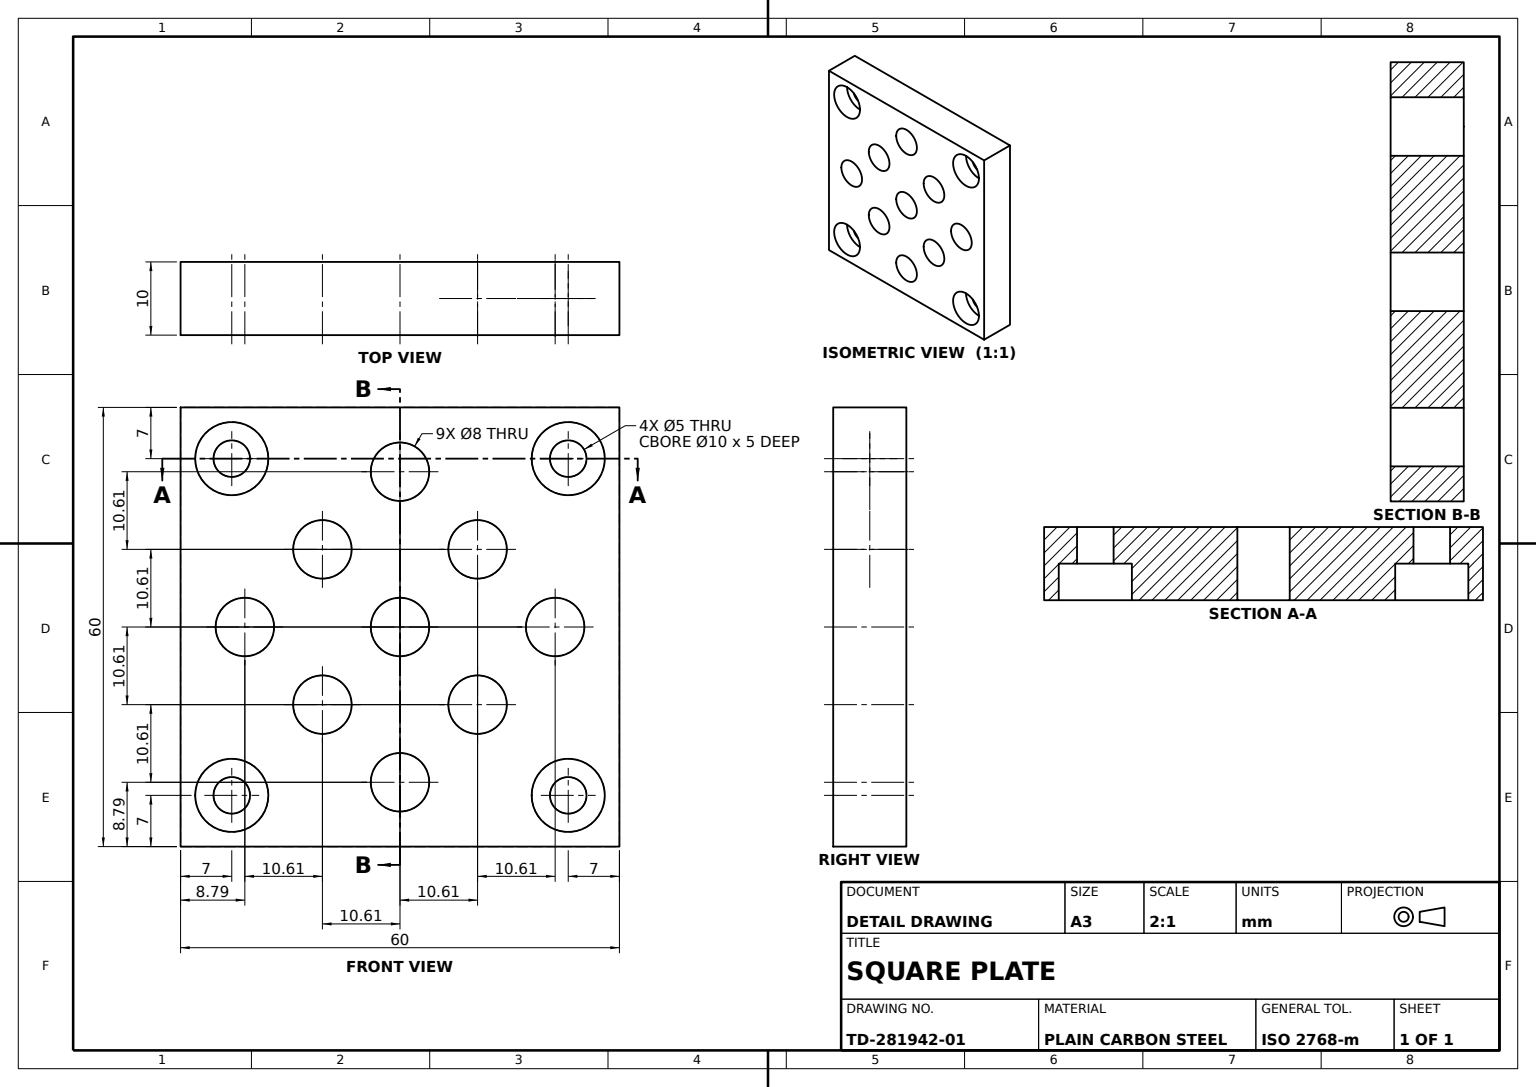
SolidWorks part; units mm, degrees
material "Plain Carbon Steel"
ref_plane "Front Plane" through (0, 0, 0) normal (0, 0, 1) x (1, 0, 0)
ref_plane "Top Plane" through (0, 0, 0) normal (0, 1, 0) x (1, 0, 0)
ref_plane "Right Plane" through (0, 0, 0) normal (1, 0, 0) x (0, 0, -1)
sketch "Plate Profile 60x60" plane through (0, 0, 0) normal (0, 0, 1) x (1, 0, 0)
  line L0 (0, 0) -> (60, 0)
  line L1 (60, 0) -> (60, 60)
  line L2 (60, 60) -> (0, 60)
  line L3 (0, 60) -> (0, 0)
  dimension "D1" = 60
  dimension "D2" = 60
  dimension "D3" = 60
extrude "Base Plate 60x60x10" add sketch "Plate Profile 60x60" along normal blind 10
sketch "Counterbore Profile 4xØ10" plane through (0, 0, 10) normal (0, 0, 1) x (1, 0, 0)
  line L0 (0, 60) -> (0, 0) construction
  line L1 (60, 60) -> (0, 60) construction
  line L2 (60, 0) -> (60, 60) construction
  line L3 (0, 0) -> (60, 0) construction
  circle A0 centre (7, 53) radius 5
  circle A1 centre (53, 53) radius 5
  circle A2 centre (7, 7) radius 5
  circle A3 centre (53, 7) radius 5
  dimension "D1" = 10
  dimension "D2" = 10
  dimension "D3" = 10
  dimension "D4" = 10
  dimension "D5" = 7
  dimension "D6" = 7
  dimension "D7" = 7
  dimension "D8" = 7
  dimension "D9" = 7
  dimension "D10" = 7
  dimension "D11" = 7
  dimension "D12" = 7
extrude "Corner Counterbores 4xØ10" cut sketch "Counterbore Profile 4xØ10" against normal blind 5
sketch "Corner Hole Profile 4xØ5" plane through (0, 0, 5) normal (0, 0, 1) x (1, 0, 0)
  circle A0 centre (7, 53) radius 2.5
  circle A1 centre (53, 53) radius 2.5
  circle A2 centre (7, 7) radius 2.5
  circle A3 centre (53, 7) radius 2.5
  dimension "D1" = 5
  dimension "D2" = 5
  dimension "D3" = 5
  dimension "D4" = 5
extrude "Corner Holes 4xØ5" cut sketch "Corner Hole Profile 4xØ5" against normal blind 5
sketch "Inner Hole Grid Profile" plane through (0, 0, 10) normal (0, 0, 1) x (1, 0, 0)
  line L0 (30, 60) -> (30, 0)
  line L1 (60, 60) -> (0, 60) construction
  line L2 (0, 0) -> (60, 0) construction
  line L3 (0, 30) -> (60, 30)
  line L4 (0, 60) -> (0, 0) construction
  line L5 (60, 0) -> (60, 60) construction
  line L6 (0, 60) -> (60, 0)
  line L7 (30, 30) -> (60, 60)
  line L8 (30, 30) -> (19.3934, 19.3934)
  line L9 (19.3934, 19.3934) -> (8.7868, 30)
  line L10 (19.3934, 19.3934) -> (30, 8.7868)
  line L11 (30, 30) -> (40.6066, 40.6066)
  line L12 (40.6066, 40.6066) -> (51.2132, 30)
  line L13 (40.6066, 40.6066) -> (30, 51.2132)
  line L14 (40.6066, 40.6066) -> (19.3934, 40.6066)
  line L15 (19.3934, 19.3934) -> (40.6066, 19.3934)
  circle A0 centre (30, 30) radius 4
  circle A1 centre (8.7868, 30) radius 4
  circle A2 centre (51.2132, 30) radius 4
  circle A3 centre (40.6066, 40.6066) radius 4
  circle A4 centre (19.3934, 19.3934) radius 4
  circle A5 centre (30, 51.2132) radius 4
  circle A6 centre (30, 8.7868) radius 4
  circle A7 centre (19.3934, 40.6066) radius 4
  circle A8 centre (40.6066, 19.3934) radius 4
  dimension "D2" = 15
  dimension "D3" = 8
  dimension "D4" = 8
  dimension "D5" = 8
  dimension "D6" = 8
  dimension "D7" = 8
  dimension "D8" = 8
  dimension "D9" = 8
  dimension "D10" = 8
  dimension "D11" = 8
  dimension "D1" = 15
extrude "Inner Through Holes 12x" cut sketch "Inner Hole Grid Profile" against normal blind 10 contours L6 A7 | L14 A7 L6 | L6 A7 L14 | L0 A5 | L13 A5 L0 | L0 A5 L13 | L13 A3 L14 | L7 A3 L13 | L12 A3 L7 | L7 A3 L12 | L14 A3 L7 | L12 A2 L3 | L3 A2 L12 | L3 A2 | L15 A8 L6 | L6 A8 | L6 A8 L15 | L9 A4 L10 | L3 A1 L9 | L3 A1 | L9 A1 L3 | L0 A6 | L10 A6 L0 | L8 A4 L9 | L15 A4 L8 | L10 A4 L15 | L6 A0 L3 | L3 A0 L7 | L7 A0 L0 | L0 A0 L6 | L6 A0 L3 | L3 A0 L8 | L8 A0 L0 | L0 A0 L6
